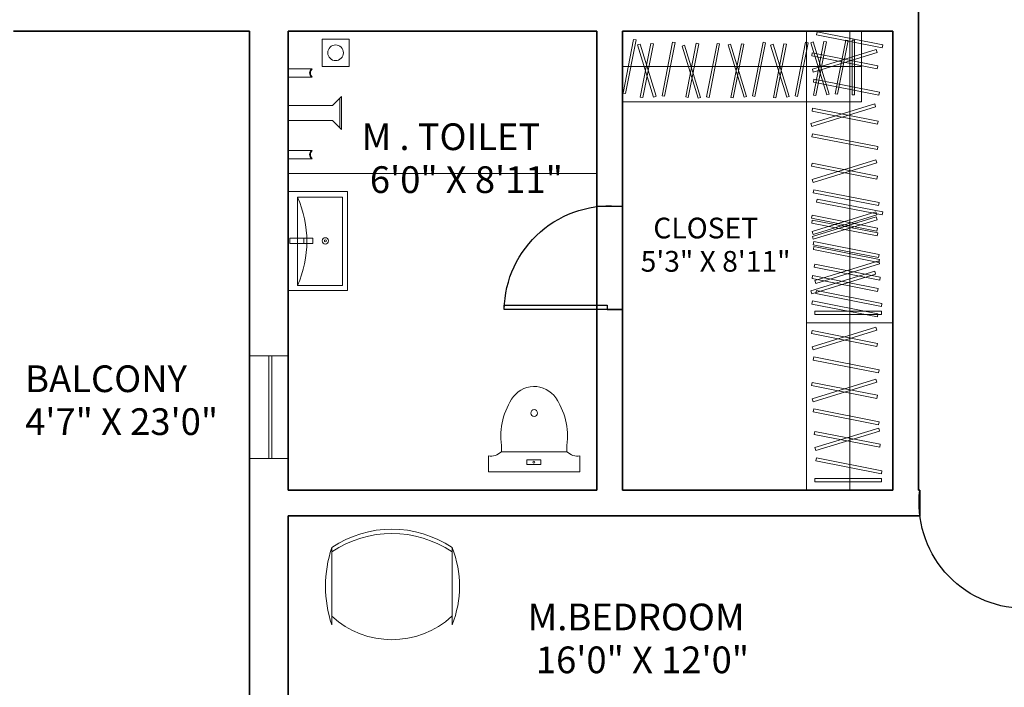
# Model space of a CAD drawing. Units: inches. Extents: x -61 to 1599, y -1316 to 257.
# Tile 191 of 204: x 1003 to 1233, y -328 to -173. Entities that reach past the tile are written whole.
import ezdxf

# ---------------------------------------------------------------- set-up
doc = ezdxf.new("R2010")
doc.units = ezdxf.units.IN
doc.header["$MEASUREMENT"] = 0
doc.linetypes.add('ACAD_ISO02W100', pattern=[15, 12, -3])
for name, color, linetype, lineweight in [('A-ANNO-DIMS', 2, 'Continuous', 18), ('A-AREA-IDEN', 1, 'Continuous', 18), ('A-FLOR-CASE', 8, 'Continuous', 18), ('A-FLOR-FIXT', 8, 'Continuous', 18), ('A-WALL-JAMB', 4, 'ACAD_ISO02W100', 25), ('DOORS', 2, 'Continuous', 25), ('FURNITURE', 83, 'Continuous', 18), ('WALLS', 4, 'Continuous', 35), ('WINDOWS', 220, 'Continuous', 18)]:
    doc.layers.add(name, color=color, linetype=linetype, lineweight=lineweight)
doc.styles.get("Standard").update_dxf_attribs({"font": 'arial.ttf'})
doc.dimstyles.get("Standard").update_dxf_attribs({"dimtxt": 0.18, "dimasz": 0.18, "dimexe": 0.18, "dimexo": 0.0625, "dimgap": 0.09, "dimtad": 0, "dimtih": 1, "dimtoh": 1, "dimdec": 0, "dimzin": 0, "dimdsep": 46, "dimlunit": 3, "dimtxsty": 'Standard', "dimcen": 0.09, "dimadec": 0, "dimazin": 0, "dimtfac": 1, "dimtdec": 0, "dimtofl": 0, "dimtmove": 0, "dimatfit": 3, "dimfxl": 1, "dimtolj": 1, "dimtzin": 0, "dimarcsym": 0})

# ---------------------------------------------------------------- blocks, each defined once
blk = doc.blocks.new('DOOR-SWING-24')
blk.add_line((0, 0), (0, 3.6))
blk.add_lwpolyline([(0, 0), (0, -24), (1.05, -24), (1.05, 0)], close=True)
blk.add_arc((-0.44, 0.62), 24.62, 271.0259, 6.9559)
blk = doc.blocks.new('WIN-24IN')
for p, q in [((0, 4.5), (0, 9)), ((0, 9), (0, 0)), ((24, 9), (24, 0)), ((0, 5.19), (24, 5.19)), ((0, 4.5), (24, 4.5))]:
    blk.add_line(p, q)
blk = doc.blocks.new('WC-FLOOR-MOUNT')
for p, q in [((3.02, 4.69), (3.02, 6.17)), ((3.02, 4.69), (18.31, 4.69)), ((18.31, 4.69), (18.31, 6.17)), ((0, 0), (0, 3.75)), ((21.33, 0), (21.33, 3.75)), ((0, 0), (21.33, 0))]:
    blk.add_line(p, q)
blk.add_lwpolyline([(12.24, 1.73), (8.96, 1.73), (8.96, 2.81), (12.24, 2.81)], close=True)
for centre, radius in [((10.67, 13.73), 0.792), ((10.6, 2.27), 0.208)]:
    blk.add_circle(centre, radius)
for centre, radius, start, end in [((10.67, 13.73), 6.18, 27.6844, 141.4697), ((19.05, 8.26), 16.17, 144.824, 187.4232), ((2.28, 8.26), 16.17, 352.5768, 35.176), ((0.56, 7.25), 3.55, 260.8586, 313.6993), ((20.77, 7.25), 3.55, 226.3007, 279.1414)]:
    blk.add_arc(centre, radius, start, end)
blk = doc.blocks.new('LAVATORY-WALL-2')
blk.add_line((3.67, 10.96), (3.67, 12.19))
for points in [[(0, 23.07), (13.87, 23.07), (13.87, 0), (0, 0)], [(12.66, 21.73), (12.66, 1.19), (2.2, 1.19), (2.2, 21.73)], [(5.78, 12.19), (5.78, 10.96), (0.4, 10.96), (0.4, 12.19)]]:
    blk.add_lwpolyline(points, close=True)
for radius in [0.74, 0.233]:
    blk.add_circle((8.7, 11.57), radius)
blk.add_arc((-20.86, 11.46), 25.25, 335.9939, 24.0061)
blk = doc.blocks.new('SHOWER-FITTINGS-3')
for p, q in [((0, 21.03), (5.62, 21.03)), ((0, 19.05), (5.62, 19.05)), ((10.34, 12.49), (12.46, 14.54)), ((12.05, 14.15), (12.05, 7.29)), ((12.46, 14.54), (12.46, 6.9)), ((0, 12.49), (10.34, 12.49)), ((0, 8.95), (10.34, 8.95)), ((10.34, 8.95), (12.46, 6.9)), ((0, 1.97), (5.62, 1.97)), ((0, 0), (5.62, 0))]:
    blk.add_line(p, q)
blk.add_lwpolyline([(14.24, 21.57), (7.95, 21.57), (7.95, 27.94), (14.24, 27.94)], close=True)
blk.add_circle((11.09, 24.76), 1.83)
for points in [[(5.44, 21.03), (5.24, 20.71), (4.83, 20.05), (5.23, 19.39), (5.44, 19.05)], [(5.62, 21.03), (5.42, 20.71), (5.02, 20.05), (5.42, 19.39), (5.62, 19.05)], [(5.44, 1.97), (5.24, 1.65), (4.83, 1), (5.23, 0.34), (5.44, 0)], [(5.62, 1.97), (5.42, 1.65), (5.02, 1), (5.42, 0.34), (5.62, 0)]]:
    blk.add_open_spline(points, degree=3, knots=[0, 0, 0, 0, 1.043806, 2.132489, 2.132489, 2.132489, 2.132489])
blk = doc.blocks.new('BEDROOM-CHAIR')
for p, q in [((1.45, 3.47), (1.45, 21.47)), ((29.49, 3.47), (29.49, 21.47))]:
    blk.add_line(p, q)
for centre, radius, start, end in [((15.47, 0.83), 24.95, 55.8098, 124.1902), ((15.47, -0.17), 24.95, 55.8098, 124.1902), ((28.58, 12.47), 28.58, 161.6455, 198.3545), ((7.26, 12.47), 23.99, 337.9646, 22.0354), ((15.47, 20.69), 20.68, 227.332, 312.668)]:
    blk.add_arc(centre, radius, start, end)
blk = doc.blocks.new('WARDROBE-HANGING')
blk.add_line((10.05, 0), (10.05, 68))
for points in [[(20.09, 0), (0, 0), (0, 68), (20.09, 68)], [(2.48, 67.85), (17.75, 64.85), (17.61, 64.14), (2.34, 67.15)], [(1.32, 62.96), (16.59, 59.95), (16.45, 59.25), (1.19, 62.25)], [(1.35, 59.16), (16.22, 63.73), (16.43, 63.04), (1.56, 58.47)], [(1.71, 56.78), (16.98, 53.78), (16.84, 53.07), (1.57, 56.08)], [(1, 46.47), (15.87, 51.04), (16.08, 50.35), (1.21, 45.78)], [(1.39, 50.01), (16.66, 47.01), (16.52, 46.3), (1.26, 49.31)], [(1.36, 44.09), (16.63, 41.09), (16.49, 40.38), (1.23, 43.38)], [(1.26, 37.2), (16.53, 34.2), (16.39, 33.49), (1.12, 36.5)], [(1.28, 33.41), (16.16, 37.98), (16.37, 37.29), (1.49, 32.72)], [(1.65, 31.03), (16.92, 28.03), (16.78, 27.32), (1.51, 30.32)], [(1.28, 21.3), (16.15, 25.87), (16.36, 25.18), (1.49, 20.61)], [(1.26, 25.09), (16.53, 22.09), (16.39, 21.38), (1.12, 24.39)], [(1.65, 18.92), (16.91, 15.92), (16.78, 15.21), (1.51, 18.21)], [(1.93, 9.89), (16.8, 14.46), (17.01, 13.77), (2.14, 9.2)], [(1.91, 13.69), (17.17, 10.68), (17.04, 9.98), (1.77, 12.98)], [(2.29, 7.51), (17.56, 4.51), (17.42, 3.8), (2.16, 6.81)], [(17.49, 1.96), (1.93, 1.96), (1.93, 2.68), (17.49, 2.68)]]:
    blk.add_lwpolyline(points, close=True)
blk = doc.blocks.new('WARDROBE-HANGING-2')
blk.add_line((55.7, 8.23), (0, 8.23))
for points in [[(55.7, 16.46), (55.7, 0), (0, 0), (0, 16.46)], [(0.12, 2.03), (2.58, 14.54), (3.16, 14.43), (0.7, 1.92)], [(9.19, 1.4), (11.65, 13.91), (12.23, 13.8), (9.77, 1.29)], [(30.28, 1.35), (32.74, 13.86), (33.32, 13.75), (30.86, 1.24)], [(40.2, 1.35), (42.66, 13.86), (43.24, 13.74), (40.78, 1.23)], [(47.6, 1.58), (43.86, 13.76), (44.42, 13.94), (48.16, 1.75)], [(44.49, 1.56), (46.95, 14.07), (47.53, 13.95), (45.07, 1.45)], [(49.55, 1.88), (52.01, 14.39), (52.59, 14.27), (50.13, 1.77)], [(54.1, 14.33), (54.1, 1.58), (53.51, 1.58), (53.51, 14.33)], [(7.24, 1.1), (3.5, 13.29), (4.06, 13.46), (7.8, 1.28)], [(4.13, 1.08), (6.59, 13.59), (7.17, 13.48), (4.71, 0.97)], [(17.64, 0.82), (13.9, 13), (14.46, 13.18), (18.2, 0.99)], [(14.73, 1.14), (17.19, 13.65), (17.77, 13.54), (15.31, 1.03)], [(19.59, 1.12), (22.05, 13.62), (22.63, 13.51), (20.17, 1)], [(28.34, 1.05), (24.59, 13.24), (25.16, 13.41), (28.9, 1.22)], [(25.23, 1.03), (27.69, 13.54), (28.27, 13.43), (25.81, 0.92)], [(38.26, 1.05), (34.51, 13.23), (35.08, 13.41), (38.82, 1.22)], [(35.15, 1.03), (37.61, 13.54), (38.19, 13.42), (35.73, 0.92)]]:
    blk.add_lwpolyline(points, close=True)
blk = doc.blocks.new('WARDROBE-HANGING-3')
blk.add_line((10.05, 0), (10.05, 68))
blk.add_lwpolyline([(20.09, 68), (20.09, 68), (20.09, 0), (0, 0), (0, 68)])
for points in [[(2.48, 67.85), (17.75, 64.85), (17.61, 64.14), (2.34, 67.15)], [(1.32, 62.96), (16.59, 59.95), (16.45, 59.25), (1.19, 62.25)], [(1.35, 59.16), (16.22, 63.73), (16.43, 63.04), (1.56, 58.47)], [(1.71, 56.78), (16.98, 53.78), (16.84, 53.07), (1.57, 56.08)], [(1, 46.47), (15.87, 51.04), (16.08, 50.35), (1.21, 45.78)], [(1.39, 50.01), (16.66, 47.01), (16.52, 46.3), (1.26, 49.31)], [(1.36, 44.09), (16.63, 41.09), (16.49, 40.38), (1.23, 43.38)], [(1.26, 37.2), (16.53, 34.2), (16.39, 33.49), (1.12, 36.5)], [(1.28, 33.41), (16.16, 37.98), (16.37, 37.29), (1.49, 32.72)], [(1.65, 31.03), (16.92, 28.03), (16.78, 27.32), (1.51, 30.32)], [(1.28, 21.3), (16.15, 25.87), (16.36, 25.18), (1.49, 20.61)], [(1.26, 25.09), (16.53, 22.09), (16.39, 21.38), (1.12, 24.39)], [(1.65, 18.92), (16.91, 15.92), (16.78, 15.21), (1.51, 18.21)], [(1.93, 9.89), (16.8, 14.46), (17.01, 13.77), (2.14, 9.2)], [(1.91, 13.69), (17.17, 10.68), (17.04, 9.98), (1.77, 12.98)], [(2.29, 7.51), (17.56, 4.51), (17.42, 3.8), (2.16, 6.81)], [(17.49, 1.96), (1.93, 1.96), (1.93, 2.68), (17.49, 2.68)]]:
    blk.add_lwpolyline(points, close=True)
blk = doc.blocks.new('*D698')
at = {"layer": 'A-ANNO-DIMS', "color": 0, "lineweight": -2, "transparency": 16777216}
for p, q in [((644.77, -167.17), (1598.48, -167.17)), ((1598.3, -167.35), (1598.3, -363.99)), ((1598.3, -560.99), (1598.3, -364.35)), ((644.77, -561.17), (1598.48, -561.17))]:
    blk.add_line(p, q, dxfattribs=at)
at = {"layer": 'A-ANNO-DIMS', "color": 0, "transparency": 16777216}
for points in [[(1598.27, -167.35), (1598.33, -167.35), (1598.3, -167.17)], [(1598.27, -560.99), (1598.33, -560.99), (1598.3, -561.17)]]:
    blk.add_solid(points, dxfattribs=at)
at = {"layer": 'DEFPOINTS', "color": 0, "transparency": 16777216}
for p in [(644.7, -167.17), (1598.3, -167.17), (644.7, -561.17)]:
    blk.add_point(p, dxfattribs=at)
at = {"layer": 'A-ANNO-DIMS', "color": 0, "transparency": 16777216, "insert": (1598.3, -364.17), "char_height": 0.18, "attachment_point": 5}
blk.add_mtext('\\A1;394', dxfattribs=at)

msp = doc.modelspace()

# ---------------------------------------------------------------- linework, layer by layer
at = {"layer": 'A-FLOR-FIXT'}
msp.add_line((1065.7028, -208.5091), (1137.7028, -208.5091), dxfattribs=at)
at = {"layer": 'A-WALL-JAMB'}
for p, q in [((1143.7028, -216.2369), (1137.7028, -216.2369)), ((1143.7028, -240.2369), (1137.7028, -240.2369)), ((1212.999, -282.3229), (1212.999, -288.3229))]:
    msp.add_line(p, q, dxfattribs=at)
at = {"layer": 'WALLS'}
for p, q in [((1212.7028, -282.3229), (1212.7028, -169.3229)), ((1001.7028, -175.3229), (1056.7028, -175.3229)), ((1056.7028, -175.3229), (1056.7028, -432.3229)), ((1065.7028, -175.3229), (1137.7028, -175.3229)), ((1065.7028, -282.3229), (1065.7028, -175.3229)), ((1137.7028, -282.3229), (1137.7028, -175.3229)), ((1143.7028, -175.3229), (1206.7028, -175.3229)), ((1143.7028, -282.3229), (1143.7028, -175.3229)), ((1206.7028, -282.3229), (1206.7028, -175.3229)), ((1065.7028, -282.3229), (1137.7028, -282.3229)), ((1143.7028, -282.3229), (1206.7028, -282.3229)), ((1212.7028, -282.3229), (1212.999, -282.3229)), ((1065.7028, -288.3229), (1065.7028, -432.3229)), ((1065.7028, -288.3229), (1213.0034, -288.3229))]:
    msp.add_line(p, q, dxfattribs=at)

# ---------------------------------------------------------------- block references
at = {"layer": 'A-FLOR-CASE'}
for name, p in [('WARDROBE-HANGING-2', (1143.703, -191.783)), ('WARDROBE-HANGING', (1186.609, -243.323)), ('WARDROBE-HANGING-3', (1186.609, -282.323))]:
    msp.add_blockref(name, p, dxfattribs=at)
at = {"layer": 'A-FLOR-FIXT'}
for name, p in [('SHOWER-FITTINGS-3', (1065.703, -205.124)), ('LAVATORY-WALL-2', (1065.703, -235.784)), ('WC-FLOOR-MOUNT', (1112.4199, -278.0925))]:
    msp.add_blockref(name, p, dxfattribs=at)
at = {"layer": 'DOORS', "extrusion": (0, 0, -1), "zscale": -1, "rotation": 90.00000000000081}
msp.add_blockref('DOOR-SWING-24', (-1140.1028, -240.2369), dxfattribs=at)
at = {"layer": 'DOORS', "extrusion": (0, 0, -1), "zscale": -1}
msp.add_blockref('DOOR-SWING-24', (-1236.999, -285.9229), dxfattribs=at)
at = {"layer": 'FURNITURE'}
msp.add_blockref('BEDROOM-CHAIR', (1074.4434, -317.2179), dxfattribs=at)
at = {"layer": 'WINDOWS', "rotation": 269.9999999999995}
msp.add_blockref('WIN-24IN', (1056.7027, -250.9933), dxfattribs=at)

# ---------------------------------------------------------------- texts
at = {"layer": 'A-AREA-IDEN'}
for s, height, p in [(' M . TOILET', 6.223643, (1080.978, -203.0507)), ('  6\'0" X 8\'11"', 6.223643, (1080.978, -213.0484)), ('  CLOSET', 4.8321, (1147.9149, -223.6457)), ('5\'3" X 8\'11"', 4.832098, (1147.9149, -231.408)), ('BALCONY', 6.22364, (1004.4051, -259.4795)), ('4\'7" X 23\'0"', 6.223643, (1004.4051, -269.4772)), ('M.BEDROOM ', 6.22364, (1121.5758, -315.0227)), (' 16\'0" X 12\'0"', 6.223643, (1121.5758, -325.0204))]:
    msp.add_text(s, height=height, dxfattribs=at).set_placement(p)

# ---------------------------------------------------------------- dimensions: what is measured, and where the dimension line sits
at = {"layer": 'A-ANNO-DIMS'}
dim = msp.add_linear_dim(base=(1598.3028, -167.169), p1=(644.7028, -561.169), p2=(644.7028, -167.169), angle=90, dimstyle='Standard', override={"dimdec": 0, "dimlfac": 1, "dimrnd": 0, "dimzin": 0, "dimdsep": 46, "dimlunit": 2}, dxfattribs=at)
dim.commit()
dim.dimension.update_dxf_attribs({"geometry": '*D698', "text_midpoint": (1598.3028, -364.169)})

doc.saveas('drawing.dxf')
